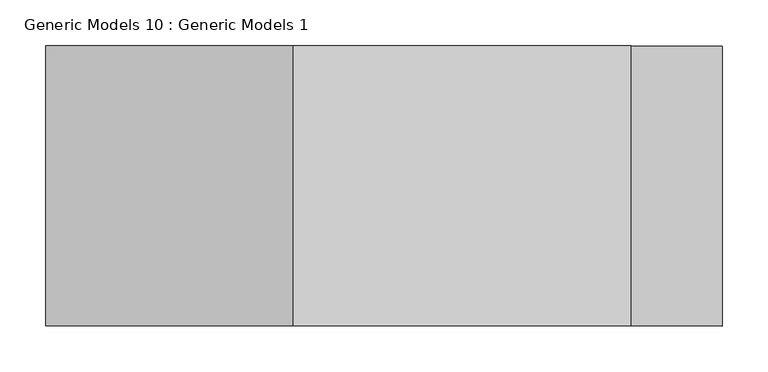
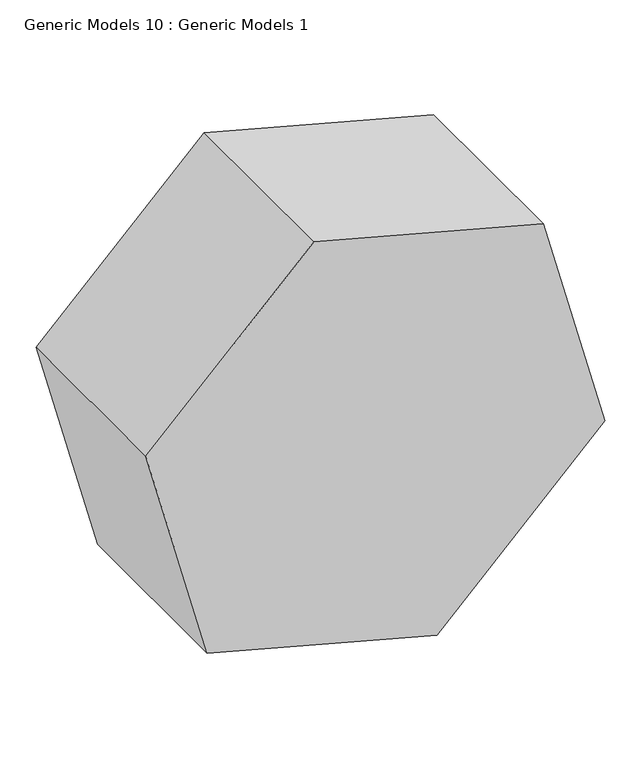
"""IFC4 building model written with IfcOpenShell, lengths in millimetres: proxy geometry, Generic Models 10 : Generic Models 1."""

from ifc_helpers import new_model, si_unit, frame, origin, place, context, project, spatial, polyline, outline, extrude, source, transform, mapped, element, save


def generic_models_10_generic_models_1_db47fcfa(model_context):
    return source(origin(), model_context, "Body", "SweptSolid", [
        extrude(outline(polyline([(904.7566299, 1506.6198357), (1003.366686, 1138.6020959), (733.9590024, 869.1944123), (365.9412626, 967.8044685), (267.3312064, 1335.8222083), (536.73889, 1605.2298919), (904.7566299, 1506.6198357)])), frame((0.0, -9086.6225464, 0.0), z_axis=(0.0, 1.0, 0.0), x_axis=(0.0, 0.0, 1.0)), (0.0, 0.0, 1.0), 304.8),
    ])


if __name__ == "__main__":
    model = new_model("IFC4")
    model_context = context("Model", 3, world=origin())
    ifc_project = project(units=[si_unit("LENGTHUNIT", "METRE", prefix="MILLI")], contexts=[model_context])
    site = spatial("IfcSite", under=ifc_project)
    building = spatial("IfcBuilding", under=site)
    placement = place(None, origin())
    generic_models_10_generic_models_1_shape = generic_models_10_generic_models_1_db47fcfa(model_context)
    element("IfcBuildingElementProxy", 1, Name="Generic Models 10 : Generic Models 1", ObjectType="Generic Models 10 : Generic Models 1", at=placement, inside=building, context=model_context, shape_type="MappedRepresentation", body=[
        mapped(generic_models_10_generic_models_1_shape, transform((0.0, 0.0, 0.0), x_axis=(1.0, 0.0, 0.0), y_axis=(0.0, 1.0, 0.0), z_axis=(0.0, 0.0, 1.0))),
    ])
    save(model, "model.ifc")

# Revit data of these elements
# Element 1 (IfcBuildingElementProxy, "Generic Models 10 : Generic Models 1")
#   Materials on its faces: "Brick, Common"
# Materials
#   "Brick, Common": class "Masonry", colour RGB 170 98 104, transparency 0, Description = "Common brick", Cost = 0
